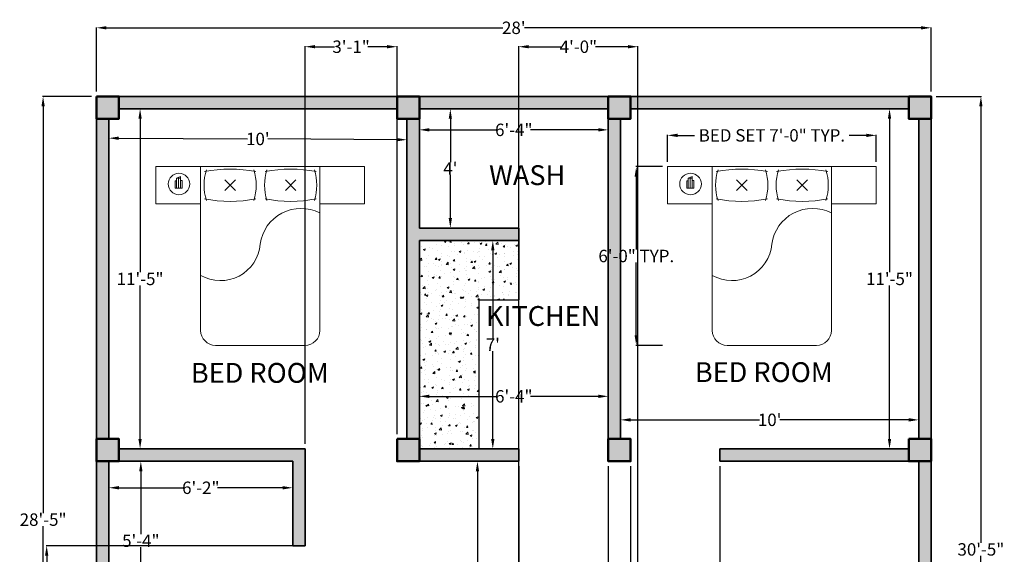
# Model space of a CAD drawing. Units: inches. Extents: x 157 to 553, y 100 to 520.
# Tile 2 of 2: x 157 to 553, y 304 to 520. Entities that reach past the tile are written whole.
import ezdxf

# ---------------------------------------------------------------- set-up
doc = ezdxf.new("R2010")
doc.units = ezdxf.units.IN
doc.header["$MEASUREMENT"] = 0
doc.layers.get('0').update_dxf_attribs({"color": 255})
for name, color, linetype, lineweight in [('A-ANNO-DIMS', 2, 'Continuous', 18), ('A-AREA-IDEN', 7, 'Continuous', 25), ('A-COLS', 7, 'Continuous', 50), ('A-FLOR-FIXT', 9, 'Continuous', 25), ('A-FLOR-FIXT-PATT', 252, 'Continuous', 13), ('A-FURN', 3, 'Continuous', 18), ('A-WALL', 7, 'Continuous', 35), ('A-WALL-PATT', 3, 'Continuous', 13)]:
    doc.layers.add(name, color=color, linetype=linetype, lineweight=lineweight)
doc.layers.add('A-COLS-PATT', color=18, linetype='Continuous', lineweight=13, true_color=0x000000)
doc.styles.get("Standard").update_dxf_attribs({"font": 'arial.ttf'})
doc.dimstyles.get("Standard").update_dxf_attribs({"dimtxt": 5, "dimasz": 4, "dimexe": 0.18, "dimexo": 2, "dimgap": 0.09, "dimtad": 0, "dimtih": 1, "dimtoh": 1, "dimdec": 0, "dimzin": 0, "dimdsep": 46, "dimlunit": 3, "dimtxsty": 'Standard', "dimcen": 2, "dimadec": 0, "dimazin": 0, "dimtfac": 1, "dimtdec": 0, "dimtofl": 0, "dimtmove": 0, "dimatfit": 3, "dimfxl": 1, "dimtolj": 1, "dimtzin": 0, "dimarcsym": 0})

# ---------------------------------------------------------------- blocks, each defined once
blk = doc.blocks.new('*D1')
at = {"layer": 'A-ANNO-DIMS', "color": 0, "lineweight": -2, "transparency": 16777216}
for p, q in [((187.79, 490.7), (187.79, 516.55)), ((191.79, 516.37), (351.41, 516.37)), ((519.79, 516.37), (360.16, 516.37)), ((523.79, 490.7), (523.79, 516.55))]:
    blk.add_line(p, q, dxfattribs=at)
at = {"layer": 'A-ANNO-DIMS', "color": 0, "transparency": 16777216}
for points in [[(191.79, 517.03), (191.79, 515.7), (187.79, 516.37)], [(519.79, 517.03), (519.79, 515.7), (523.79, 516.37)]]:
    blk.add_solid(points, dxfattribs=at)
at = {"layer": 'Defpoints', "color": 0, "transparency": 16777216}
for p in [(523.79, 516.37), (187.79, 488.7), (523.79, 488.7)]:
    blk.add_point(p, dxfattribs=at)
at = {"layer": 'A-ANNO-DIMS', "color": 0, "transparency": 16777216, "insert": (355.79, 516.37), "char_height": 5, "attachment_point": 5}
blk.add_mtext("\\A1;28'", dxfattribs=at)
blk = doc.blocks.new('*D2')
at = {"layer": 'A-ANNO-DIMS', "color": 0, "lineweight": -2, "transparency": 16777216}
for p, q in [((185.79, 488.7), (166.12, 488.7)), ((166.3, 484.7), (166.3, 320.85)), ((166.3, 151.7), (166.3, 315.56)), ((185.79, 147.7), (166.12, 147.7))]:
    blk.add_line(p, q, dxfattribs=at)
at = {"layer": 'A-ANNO-DIMS', "color": 0, "transparency": 16777216}
for points in [[(165.64, 484.7), (166.97, 484.7), (166.3, 488.7)], [(165.64, 151.7), (166.97, 151.7), (166.3, 147.7)]]:
    blk.add_solid(points, dxfattribs=at)
at = {"layer": 'Defpoints', "color": 0, "transparency": 16777216}
for p in [(187.79, 488.7), (166.3, 147.7), (187.79, 147.7)]:
    blk.add_point(p, dxfattribs=at)
at = {"layer": 'A-ANNO-DIMS', "color": 0, "transparency": 16777216, "insert": (166.3, 318.2), "char_height": 5, "attachment_point": 5}
blk.add_mtext('\\A1;28\'-5"', dxfattribs=at)
blk = doc.blocks.new('*D4')
at = {"layer": 'A-ANNO-DIMS', "color": 0, "lineweight": -2, "transparency": 16777216}
for p, q in [((512.79, 483.7), (506.88, 483.7)), ((507.06, 479.7), (507.06, 417.85)), ((507.06, 350.7), (507.06, 412.56)), ((512.79, 346.7), (506.88, 346.7))]:
    blk.add_line(p, q, dxfattribs=at)
at = {"layer": 'A-ANNO-DIMS', "color": 0, "transparency": 16777216}
for points in [[(506.39, 479.7), (507.72, 479.7), (507.06, 483.7)], [(506.39, 350.7), (507.72, 350.7), (507.06, 346.7)]]:
    blk.add_solid(points, dxfattribs=at)
at = {"layer": 'Defpoints', "color": 0, "transparency": 16777216}
for p in [(514.79, 483.7), (507.06, 346.7), (514.79, 346.7)]:
    blk.add_point(p, dxfattribs=at)
at = {"layer": 'A-ANNO-DIMS', "color": 0, "transparency": 16777216, "insert": (507.06, 415.2), "char_height": 5, "attachment_point": 5}
blk.add_mtext('\\A1;11\'-5"', dxfattribs=at)
blk = doc.blocks.new('*D5')
at = {"layer": 'A-ANNO-DIMS', "color": 0, "lineweight": -2, "transparency": 16777216}
for p, q in [((398.79, 352.7), (398.79, 358.58)), ((402.79, 358.4), (454.69, 358.4)), ((514.79, 358.4), (462.89, 358.4)), ((518.79, 352.7), (518.79, 358.58))]:
    blk.add_line(p, q, dxfattribs=at)
at = {"layer": 'A-ANNO-DIMS', "color": 0, "transparency": 16777216}
for points in [[(402.79, 359.07), (402.79, 357.73), (398.79, 358.4)], [(514.79, 359.07), (514.79, 357.73), (518.79, 358.4)]]:
    blk.add_solid(points, dxfattribs=at)
at = {"layer": 'Defpoints', "color": 0, "transparency": 16777216}
for p in [(518.79, 358.4), (398.79, 350.7), (518.79, 350.7)]:
    blk.add_point(p, dxfattribs=at)
at = {"layer": 'A-ANNO-DIMS', "color": 0, "transparency": 16777216, "insert": (458.79, 358.4), "char_height": 5, "attachment_point": 5}
blk.add_mtext("\\A1;10'", dxfattribs=at)
blk = doc.blocks.new('*D6')
at = {"layer": 'A-ANNO-DIMS', "color": 0, "lineweight": -2, "transparency": 16777216}
for p, q in [((198.79, 483.7), (205.52, 483.7)), ((205.34, 479.7), (205.34, 417.85)), ((205.34, 350.7), (205.34, 412.56)), ((198.79, 346.7), (205.52, 346.7))]:
    blk.add_line(p, q, dxfattribs=at)
at = {"layer": 'A-ANNO-DIMS', "color": 0, "transparency": 16777216}
for points in [[(204.67, 479.7), (206.01, 479.7), (205.34, 483.7)], [(204.67, 350.7), (206.01, 350.7), (205.34, 346.7)]]:
    blk.add_solid(points, dxfattribs=at)
at = {"layer": 'Defpoints', "color": 0, "transparency": 16777216}
for p in [(196.79, 483.7), (196.79, 346.7), (205.34, 346.7)]:
    blk.add_point(p, dxfattribs=at)
at = {"layer": 'A-ANNO-DIMS', "color": 0, "transparency": 16777216, "insert": (205.34, 415.2), "char_height": 5, "attachment_point": 5}
blk.add_mtext('\\A1;11\'-5"', dxfattribs=at)
blk = doc.blocks.new('*D7')
at = {"layer": 'A-ANNO-DIMS', "color": 0, "lineweight": -2, "transparency": 16777216}
for p, q in [((192.78, 477.7), (192.75, 471.72)), ((312.78, 477.08), (312.75, 471.09)), ((196.75, 471.88), (248.65, 471.61)), ((308.75, 471.3), (256.84, 471.57))]:
    blk.add_line(p, q, dxfattribs=at)
at = {"layer": 'A-ANNO-DIMS', "color": 0, "transparency": 16777216}
for points in [[(196.75, 472.55), (196.74, 471.21), (192.75, 471.9)], [(308.75, 471.96), (308.74, 470.63), (312.75, 471.27)]]:
    blk.add_solid(points, dxfattribs=at)
at = {"layer": 'Defpoints', "color": 0, "transparency": 16777216}
for p in [(192.79, 479.7), (312.79, 479.08), (312.75, 471.27)]:
    blk.add_point(p, dxfattribs=at)
at = {"layer": 'A-ANNO-DIMS', "color": 0, "transparency": 16777216, "insert": (252.75, 471.59), "char_height": 5, "attachment_point": 5}
blk.add_mtext("\\A1;10'", dxfattribs=at)
blk = doc.blocks.new('*D8')
at = {"layer": 'A-ANNO-DIMS', "color": 0, "lineweight": -2, "transparency": 16777216}
for p, q in [((317.79, 477.7), (317.79, 475.08)), ((393.79, 477.7), (393.79, 475.08)), ((321.79, 475.26), (349.04, 475.26)), ((389.79, 475.26), (362.54, 475.26))]:
    blk.add_line(p, q, dxfattribs=at)
at = {"layer": 'A-ANNO-DIMS', "color": 0, "transparency": 16777216}
for points in [[(321.79, 475.93), (321.79, 474.59), (317.79, 475.26)], [(389.79, 475.93), (389.79, 474.59), (393.79, 475.26)]]:
    blk.add_solid(points, dxfattribs=at)
at = {"layer": 'Defpoints', "color": 0, "transparency": 16777216}
for p in [(317.79, 479.7), (393.79, 479.7), (393.79, 475.26)]:
    blk.add_point(p, dxfattribs=at)
at = {"layer": 'A-ANNO-DIMS', "color": 0, "transparency": 16777216, "insert": (355.79, 475.26), "char_height": 5, "attachment_point": 5}
blk.add_mtext('\\A1;6\'-4"', dxfattribs=at)
blk = doc.blocks.new('*D9')
at = {"layer": 'A-ANNO-DIMS', "color": 0, "lineweight": -2, "transparency": 16777216}
for p, q in [((319.79, 483.7), (330.43, 483.7)), ((330.25, 479.7), (330.25, 462.29)), ((330.25, 439.7), (330.25, 457.11)), ((319.79, 435.7), (330.43, 435.7))]:
    blk.add_line(p, q, dxfattribs=at)
at = {"layer": 'A-ANNO-DIMS', "color": 0, "transparency": 16777216}
for points in [[(329.58, 479.7), (330.91, 479.7), (330.25, 483.7)], [(329.58, 439.7), (330.91, 439.7), (330.25, 435.7)]]:
    blk.add_solid(points, dxfattribs=at)
at = {"layer": 'Defpoints', "color": 0, "transparency": 16777216}
for p in [(317.79, 483.7), (330.25, 483.7), (317.79, 435.7)]:
    blk.add_point(p, dxfattribs=at)
at = {"layer": 'A-ANNO-DIMS', "color": 0, "transparency": 16777216, "insert": (330.25, 459.7), "char_height": 5, "attachment_point": 5}
blk.add_mtext("\\A1;4'", dxfattribs=at)
blk = doc.blocks.new('*D10')
at = {"layer": 'A-ANNO-DIMS', "color": 0, "lineweight": -2, "transparency": 16777216}
for p, q in [((339.59, 430.7), (347.52, 430.7)), ((347.34, 426.7), (347.34, 391.29)), ((347.34, 350.7), (347.34, 386.11)), ((339.59, 346.7), (347.52, 346.7))]:
    blk.add_line(p, q, dxfattribs=at)
at = {"layer": 'A-ANNO-DIMS', "color": 0, "transparency": 16777216}
for points in [[(346.67, 426.7), (348, 426.7), (347.34, 430.7)], [(346.67, 350.7), (348, 350.7), (347.34, 346.7)]]:
    blk.add_solid(points, dxfattribs=at)
at = {"layer": 'Defpoints', "color": 0, "transparency": 16777216}
for p in [(337.59, 430.7), (347.34, 430.7), (337.59, 346.7)]:
    blk.add_point(p, dxfattribs=at)
at = {"layer": 'A-ANNO-DIMS', "color": 0, "transparency": 16777216, "insert": (347.34, 388.7), "char_height": 5, "attachment_point": 5}
blk.add_mtext("\\A1;7'", dxfattribs=at)
blk = doc.blocks.new('*D11')
at = {"layer": 'A-ANNO-DIMS', "color": 0, "lineweight": -2, "transparency": 16777216}
for p, q in [((317.79, 375.65), (317.79, 367.7)), ((393.79, 375.65), (393.79, 367.7)), ((321.79, 367.88), (349.04, 367.88)), ((389.79, 367.88), (362.54, 367.88))]:
    blk.add_line(p, q, dxfattribs=at)
at = {"layer": 'A-ANNO-DIMS', "color": 0, "transparency": 16777216}
for points in [[(321.79, 368.55), (321.79, 367.21), (317.79, 367.88)], [(389.79, 368.55), (389.79, 367.21), (393.79, 367.88)]]:
    blk.add_solid(points, dxfattribs=at)
at = {"layer": 'Defpoints', "color": 0, "transparency": 16777216}
for p in [(317.79, 377.65), (393.79, 377.65), (393.79, 367.88)]:
    blk.add_point(p, dxfattribs=at)
at = {"layer": 'A-ANNO-DIMS', "color": 0, "transparency": 16777216, "insert": (355.79, 367.88), "char_height": 5, "attachment_point": 5}
blk.add_mtext('\\A1;6\'-4"', dxfattribs=at)
blk = doc.blocks.new('*D12')
at = {"layer": 'A-ANNO-DIMS', "color": 0, "lineweight": -2, "transparency": 16777216}
for p, q in [((192.79, 339.7), (192.79, 330.86)), ((266.79, 339.7), (266.79, 330.86)), ((196.79, 331.04), (223.04, 331.04)), ((262.79, 331.04), (236.54, 331.04))]:
    blk.add_line(p, q, dxfattribs=at)
at = {"layer": 'A-ANNO-DIMS', "color": 0, "transparency": 16777216}
for points in [[(196.79, 331.71), (196.79, 330.37), (192.79, 331.04)], [(262.79, 331.71), (262.79, 330.37), (266.79, 331.04)]]:
    blk.add_solid(points, dxfattribs=at)
at = {"layer": 'Defpoints', "color": 0, "transparency": 16777216}
for p in [(192.79, 341.7), (266.79, 341.7), (266.79, 331.04)]:
    blk.add_point(p, dxfattribs=at)
at = {"layer": 'A-ANNO-DIMS', "color": 0, "transparency": 16777216, "insert": (229.79, 331.04), "char_height": 5, "attachment_point": 5}
blk.add_mtext('\\A1;6\'-2"', dxfattribs=at)
blk = doc.blocks.new('*D13')
at = {"layer": 'A-ANNO-DIMS', "color": 0, "lineweight": -2, "transparency": 16777216}
for p, q in [((198.79, 341.7), (205.83, 341.7)), ((205.65, 337.7), (205.65, 312.34)), ((205.65, 281.7), (205.65, 307.07)), ((198.79, 277.7), (205.83, 277.7))]:
    blk.add_line(p, q, dxfattribs=at)
at = {"layer": 'A-ANNO-DIMS', "color": 0, "transparency": 16777216}
for points in [[(204.99, 337.7), (206.32, 337.7), (205.65, 341.7)], [(204.99, 281.7), (206.32, 281.7), (205.65, 277.7)]]:
    blk.add_solid(points, dxfattribs=at)
at = {"layer": 'Defpoints', "color": 0, "transparency": 16777216}
for p in [(196.79, 341.7), (196.79, 277.7), (205.65, 277.7)]:
    blk.add_point(p, dxfattribs=at)
at = {"layer": 'A-ANNO-DIMS', "color": 0, "transparency": 16777216, "insert": (205.65, 309.7), "char_height": 5, "attachment_point": 5}
blk.add_mtext('\\A1;5\'-4"', dxfattribs=at)
blk = doc.blocks.new('*D18')
at = {"layer": 'A-ANNO-DIMS', "color": 0, "lineweight": -2, "transparency": 16777216}
for p, q in [((355.79, 341.7), (340.98, 341.7)), ((341.16, 337.7), (341.16, 285.85)), ((341.16, 228.7), (341.16, 280.56)), ((355.79, 224.7), (340.98, 224.7))]:
    blk.add_line(p, q, dxfattribs=at)
at = {"layer": 'A-ANNO-DIMS', "color": 0, "transparency": 16777216}
for points in [[(340.49, 337.7), (341.82, 337.7), (341.16, 341.7)], [(340.49, 228.7), (341.82, 228.7), (341.16, 224.7)]]:
    blk.add_solid(points, dxfattribs=at)
at = {"layer": 'Defpoints', "color": 0, "transparency": 16777216}
for p in [(341.16, 341.7), (357.79, 341.7), (357.79, 224.7)]:
    blk.add_point(p, dxfattribs=at)
at = {"layer": 'A-ANNO-DIMS', "color": 0, "transparency": 16777216, "insert": (341.16, 283.2), "char_height": 5, "attachment_point": 5}
blk.add_mtext('\\A1;9\'-9"', dxfattribs=at)
blk = doc.blocks.new('BED-DOUBLE-WITH-NIGHTSTANDS')
for p, q in [((0, 72), (18, 72)), ((0, 57), (0, 72)), ((6, 72), (84, 72)), ((18, 72), (18, 6)), ((66, 6), (66, 72)), ((84, 72), (84, 57)), ((9.95, 67.98), (8.32, 67.38)), ((9.95, 67.38), (9.95, 67.98)), ((9.14, 67.38), (9.14, 63.35)), ((32, 66.63), (27.75, 62.4)), ((27.76, 66.64), (31.99, 62.39)), ((56.35, 66.63), (52.1, 62.4)), ((52.11, 66.64), (56.34, 62.39)), ((18, 57), (0, 57)), ((84, 57), (66, 57)), ((24, 0), (60, 0))]:
    blk.add_line(p, q)
for points in [[(8.32, 63.35), (7.8, 63.35), (7.8, 66.31), (8.32, 66.31)], [(8.32, 63.35), (9.95, 63.35), (9.95, 67.38), (8.32, 67.38)], [(9.95, 63.35), (10.59, 63.35), (10.59, 66.42), (9.95, 66.42)]]:
    blk.add_lwpolyline(points, close=True)
blk.add_circle((9.27, 65.01), 4.35)
for centre, radius, start, end in [((54.23, 16.39), 56.63, 100.869, 100.8807), ((54.23, 16.39), 56.63, 79.1193, 79.131), ((40, 64.52), 20.63, 162.5077, 197.4923), ((29.88, 16.39), 54.63, 79.1193, 100.8807), ((19.75, 64.52), 20.62, 342.5077, 17.4923), ((64.35, 64.52), 20.63, 162.5077, 197.4923), ((54.23, 16.39), 54.63, 79.1193, 100.8807), ((44.1, 64.52), 20.62, 342.5077, 17.4923), ((29.88, 112.64), 54.63, 259.1193, 280.8807), ((54.23, 112.64), 54.63, 259.1193, 280.8807), ((58.39, 38.66), 16.52, 62.5747, 172.7011), ((25.97, 42.18), 16.1, 240.3431, 354.9328), ((24, 6), 6, 180, 270), ((60, 6), 6, 270, 0)]:
    blk.add_arc(centre, radius, start, end)
blk = doc.blocks.new('*D21')
at = {"layer": 'A-ANNO-DIMS', "color": 0, "lineweight": -2, "transparency": 16777216}
for p, q in [((417.7, 462.43), (417.7, 473.21)), ((421.7, 473.03), (428.56, 473.03)), ((497.7, 473.03), (490.83, 473.03)), ((501.7, 462.43), (501.7, 473.21))]:
    blk.add_line(p, q, dxfattribs=at)
at = {"layer": 'A-ANNO-DIMS', "color": 0, "transparency": 16777216}
for points in [[(421.7, 473.7), (421.7, 472.36), (417.7, 473.03)], [(497.7, 473.7), (497.7, 472.36), (501.7, 473.03)]]:
    blk.add_solid(points, dxfattribs=at)
at = {"layer": 'Defpoints', "color": 0, "transparency": 16777216}
for p in [(501.7, 473.03), (417.7, 460.43), (501.7, 460.43)]:
    blk.add_point(p, dxfattribs=at)
at = {"layer": 'A-ANNO-DIMS', "color": 0, "transparency": 16777216, "insert": (459.7, 473.03), "char_height": 5, "attachment_point": 5}
blk.add_mtext('\\A1;BED SET 7\'-0" TYP.', dxfattribs=at)
blk = doc.blocks.new('*D22')
at = {"layer": 'A-ANNO-DIMS', "color": 0, "lineweight": -2, "transparency": 16777216}
for p, q in [((415.7, 460.43), (404.92, 460.43)), ((405.1, 456.43), (405.1, 427.07)), ((405.1, 392.43), (405.1, 421.79)), ((415.7, 388.43), (404.92, 388.43))]:
    blk.add_line(p, q, dxfattribs=at)
at = {"layer": 'A-ANNO-DIMS', "color": 0, "transparency": 16777216}
for points in [[(404.43, 456.43), (405.76, 456.43), (405.1, 460.43)], [(404.43, 392.43), (405.76, 392.43), (405.1, 388.43)]]:
    blk.add_solid(points, dxfattribs=at)
at = {"layer": 'Defpoints', "color": 0, "transparency": 16777216}
for p in [(405.1, 460.43), (417.7, 460.43), (417.7, 388.43)]:
    blk.add_point(p, dxfattribs=at)
at = {"layer": 'A-ANNO-DIMS', "color": 0, "transparency": 16777216, "insert": (405.1, 424.43), "char_height": 5, "attachment_point": 5}
blk.add_mtext('\\A1;6\'-0" TYP.', dxfattribs=at)
blk = doc.blocks.new('*D23')
at = {"layer": 'A-ANNO-DIMS', "color": 0, "lineweight": -2, "transparency": 16777216}
for p, q in [((525.79, 488.7), (544.02, 488.7)), ((543.84, 484.7), (543.84, 308.85)), ((543.84, 127.7), (543.84, 303.56)), ((406.79, 123.7), (544.02, 123.7))]:
    blk.add_line(p, q, dxfattribs=at)
at = {"layer": 'A-ANNO-DIMS', "color": 0, "transparency": 16777216}
for points in [[(543.17, 484.7), (544.5, 484.7), (543.84, 488.7)], [(543.17, 127.7), (544.5, 127.7), (543.84, 123.7)]]:
    blk.add_solid(points, dxfattribs=at)
at = {"layer": 'Defpoints', "color": 0, "transparency": 16777216}
for p in [(523.79, 488.7), (404.79, 123.7), (543.84, 123.7)]:
    blk.add_point(p, dxfattribs=at)
at = {"layer": 'A-ANNO-DIMS', "color": 0, "transparency": 16777216, "insert": (543.84, 306.2), "char_height": 5, "attachment_point": 5}
blk.add_mtext('\\A1;30\'-5"', dxfattribs=at)
blk = doc.blocks.new('*D24')
at = {"layer": 'A-ANNO-DIMS', "color": 0, "lineweight": -2, "transparency": 16777216}
for p, q in [((271.79, 348.7), (271.79, 508.93)), ((275.79, 508.75), (283.55, 508.75)), ((304.79, 508.75), (297.02, 508.75)), ((308.79, 352.7), (308.79, 508.93))]:
    blk.add_line(p, q, dxfattribs=at)
at = {"layer": 'A-ANNO-DIMS', "color": 0, "transparency": 16777216}
for points in [[(275.79, 509.42), (275.79, 508.09), (271.79, 508.75)], [(304.79, 509.42), (304.79, 508.09), (308.79, 508.75)]]:
    blk.add_solid(points, dxfattribs=at)
at = {"layer": 'Defpoints', "color": 0, "transparency": 16777216}
for p in [(308.79, 508.75), (308.79, 350.7), (271.79, 346.7)]:
    blk.add_point(p, dxfattribs=at)
at = {"layer": 'A-ANNO-DIMS', "color": 0, "transparency": 16777216, "insert": (290.29, 508.75), "char_height": 5, "attachment_point": 5}
blk.add_mtext('\\A1;3\'-1"', dxfattribs=at)
blk = doc.blocks.new('*D25')
at = {"layer": 'A-ANNO-DIMS', "color": 0, "lineweight": -2, "transparency": 16777216}
for p, q in [((357.79, 339.7), (357.79, 103.47)), ((393.79, 339.7), (393.79, 103.47)), ((361.79, 103.65), (369.05, 103.65)), ((389.79, 103.65), (382.52, 103.65))]:
    blk.add_line(p, q, dxfattribs=at)
at = {"layer": 'A-ANNO-DIMS', "color": 0, "transparency": 16777216}
for points in [[(361.79, 104.32), (361.79, 102.99), (357.79, 103.65)], [(389.79, 104.32), (389.79, 102.99), (393.79, 103.65)]]:
    blk.add_solid(points, dxfattribs=at)
at = {"layer": 'Defpoints', "color": 0, "transparency": 16777216}
for p in [(357.79, 341.7), (393.79, 341.7), (393.79, 103.65)]:
    blk.add_point(p, dxfattribs=at)
at = {"layer": 'A-ANNO-DIMS', "color": 0, "transparency": 16777216, "insert": (375.79, 103.65), "char_height": 5, "attachment_point": 5}
blk.add_mtext('\\A1;3\'-0"', dxfattribs=at)
blk = doc.blocks.new('*D26')
at = {"layer": 'A-ANNO-DIMS', "color": 0, "lineweight": -2, "transparency": 16777216}
for p, q in [((402.79, 339.7), (402.79, 103.47)), ((438.79, 339.7), (438.79, 103.47)), ((406.79, 103.65), (414.05, 103.65)), ((434.79, 103.65), (427.52, 103.65))]:
    blk.add_line(p, q, dxfattribs=at)
at = {"layer": 'A-ANNO-DIMS', "color": 0, "transparency": 16777216}
for points in [[(406.79, 104.32), (406.79, 102.99), (402.79, 103.65)], [(434.79, 104.32), (434.79, 102.99), (438.79, 103.65)]]:
    blk.add_solid(points, dxfattribs=at)
at = {"layer": 'Defpoints', "color": 0, "transparency": 16777216}
for p in [(402.79, 341.7), (438.79, 341.7), (438.79, 103.65)]:
    blk.add_point(p, dxfattribs=at)
at = {"layer": 'A-ANNO-DIMS', "color": 0, "transparency": 16777216, "insert": (420.79, 103.65), "char_height": 5, "attachment_point": 5}
blk.add_mtext('\\A1;3\'-0"', dxfattribs=at)
blk = doc.blocks.new('*D27')
at = {"layer": 'A-ANNO-DIMS', "color": 0, "lineweight": -2, "transparency": 16777216}
for p, q in [((269.79, 307.7), (167.56, 307.7)), ((167.74, 303.7), (167.74, 295.35)), ((167.74, 281.7), (167.74, 290.06)), ((306.79, 277.7), (167.56, 277.7))]:
    blk.add_line(p, q, dxfattribs=at)
at = {"layer": 'A-ANNO-DIMS', "color": 0, "transparency": 16777216}
for points in [[(167.07, 303.7), (168.4, 303.7), (167.74, 307.7)], [(167.07, 281.7), (168.4, 281.7), (167.74, 277.7)]]:
    blk.add_solid(points, dxfattribs=at)
at = {"layer": 'Defpoints', "color": 0, "transparency": 16777216}
for p in [(271.79, 307.7), (167.74, 277.7), (308.79, 277.7)]:
    blk.add_point(p, dxfattribs=at)
at = {"layer": 'A-ANNO-DIMS', "color": 0, "transparency": 16777216, "insert": (167.74, 292.7), "char_height": 5, "attachment_point": 5}
blk.add_mtext('\\A1;2\'-6"', dxfattribs=at)
blk = doc.blocks.new('*D29')
at = {"layer": 'A-ANNO-DIMS', "color": 0, "lineweight": -2, "transparency": 16777216}
for p, q in [((357.79, 226.7), (357.79, 508.93)), ((361.79, 508.75), (374.95, 508.75)), ((401.79, 508.75), (388.62, 508.75)), ((405.79, 226.7), (405.79, 508.93))]:
    blk.add_line(p, q, dxfattribs=at)
at = {"layer": 'A-ANNO-DIMS', "color": 0, "transparency": 16777216}
for points in [[(361.79, 509.42), (361.79, 508.09), (357.79, 508.75)], [(401.79, 509.42), (401.79, 508.09), (405.79, 508.75)]]:
    blk.add_solid(points, dxfattribs=at)
at = {"layer": 'Defpoints', "color": 0, "transparency": 16777216}
for p in [(405.79, 508.75), (357.79, 224.7), (405.79, 224.7)]:
    blk.add_point(p, dxfattribs=at)
at = {"layer": 'A-ANNO-DIMS', "color": 0, "transparency": 16777216, "insert": (381.79, 508.75), "char_height": 5, "attachment_point": 5}
blk.add_mtext('\\A1;4\'-0"', dxfattribs=at)

msp = doc.modelspace()

# ---------------------------------------------------------------- hatches: boundary and pattern name
at = {"layer": 'A-COLS-PATT'}
h = msp.add_hatch(color=256, dxfattribs=at)
h.dxf.hatch_style = 1
h.paths.add_polyline_path([(196.79, 156.7), (187.79, 156.7), (187.79, 147.7), (196.79, 147.7)])
h.paths.add_polyline_path([(317.79, 156.7), (308.79, 156.7), (308.79, 147.7), (317.79, 147.7)])
h.paths.add_polyline_path([(440.79, 156.7), (431.79, 156.7), (431.79, 147.7), (440.79, 147.7)])
h.paths.add_polyline_path([(523.79, 156.7), (514.79, 156.7), (514.79, 147.7), (523.79, 147.7)])
h.paths.add_polyline_path([(523.79, 277.7), (514.79, 277.7), (514.79, 268.7), (523.79, 268.7)])
h.paths.add_polyline_path([(440.79, 277.7), (431.79, 277.7), (431.79, 268.7), (440.79, 268.7)])
h.paths.add_polyline_path([(317.79, 277.7), (308.79, 277.7), (308.79, 268.7), (317.79, 268.7)])
h.paths.add_polyline_path([(196.79, 350.7), (187.79, 350.7), (187.79, 341.7), (196.79, 341.7)])
h.paths.add_polyline_path([(317.79, 350.7), (308.79, 350.7), (308.79, 341.7), (317.79, 341.7)])
h.paths.add_polyline_path([(402.79, 350.7), (393.79, 350.7), (393.79, 341.7), (402.79, 341.7)])
h.paths.add_polyline_path([(523.79, 350.7), (514.79, 350.7), (514.79, 341.7), (523.79, 341.7)])
h.paths.add_polyline_path([(523.79, 488.7), (514.79, 488.7), (514.79, 479.7), (523.79, 479.7)])
h.paths.add_polyline_path([(402.79, 488.7), (393.79, 488.7), (393.79, 479.7), (402.79, 479.7)])
h.paths.add_polyline_path([(317.79, 488.7), (308.79, 488.7), (308.79, 479.7), (317.79, 479.7)])
h.paths.add_polyline_path([(196.79, 488.7), (187.79, 488.7), (187.79, 479.7), (196.79, 479.7)])
at = {"layer": 'A-FLOR-FIXT-PATT'}
h = msp.add_hatch(dxfattribs=at)
h.set_pattern_fill('AR-CONC', color=256)
h.set_pattern_definition([(50, (0, 0), (7.1726, -0.62752), [0.75, -8.25]), (355, (0, 0), (-1.38751, 7.52192), [0.6, -6.6]), (100.4514, (0.598, -0.052), (5.78509, 6.8944), [0.6374, -7.01142]), (46.1842, (0, 2), (10.67241, -1.65519), [1.125, -12.375]), (96.6356, (0.889, 1.862), (9.34662, 9.74119), [0.9561, -10.51714]), (351.1842, (0, 2), (9.34662, 9.74119), [0.9, -9.9]), (21, (1, 1.5), (5.96907, -4.02619), [0.75, -8.25]), (326, (1, 1.5), (2.43315, 7.2515), [0.6, -6.6]), (71.4514, (1.4974, 1.1645), (8.40222, 3.22531), [0.6374, -7.01142]), (37.5, (0, 0), (0.121599, 3.328939), [0, -6.52, 0, -6.7, 0, -6.625]), (7.5, (0, 0), (2.630695, 3.944117), [0, -3.82, 0, -6.37, 0, -2.525]), (327.5, (-2.23, 0), (5.338224, -0.225549), [0, -2.5, 0, -7.8, 0, -10.35]), (317.5, (-3.23, 0), (5.83186, 1.00105), [0, -3.25, 0, -5.18, 0, -7.35])])
h.paths.add_polyline_path([(357.79, 430.7), (317.79, 430.7), (317.79, 346.7), (341.79, 346.7), (341.79, 406.7), (357.79, 406.7)])
at = {"layer": 'A-WALL-PATT'}
h = msp.add_hatch(color=256, dxfattribs=at)
h.dxf.hatch_style = 1
h.paths.add_polyline_path([(271.79, 346.7), (196.79, 346.7), (196.79, 341.7), (266.79, 341.7), (266.79, 307.7), (271.79, 307.7)])
h.paths.add_polyline_path([(308.79, 277.7), (192.79, 277.7), (192.79, 341.7), (187.79, 341.7), (187.79, 156.7), (192.79, 156.7), (192.79, 272.7), (308.79, 272.7)])
h.paths.add_polyline_path([(357.79, 224.7), (317.79, 224.7), (317.79, 232.7), (312.79, 232.7), (312.79, 156.7), (317.79, 156.7), (317.79, 219.7), (357.79, 219.7)])
h.paths.add_polyline_path([(308.79, 152.7), (196.79, 152.7), (196.79, 147.7), (308.79, 147.7)])
h.paths.add_polyline_path([(440.79, 268.7), (435.79, 268.7), (435.79, 224.7), (405.79, 224.7), (405.79, 219.7), (435.79, 219.7), (435.79, 156.7), (440.79, 156.7)])
h.paths.add_polyline_path([(523.79, 147.7), (518.79, 147.7), (518.79, 131.7), (440.79, 131.7), (440.79, 147.7), (435.79, 147.7), (435.79, 126.7), (523.79, 126.7)])
h.paths.add_polyline_path([(523.79, 268.7), (518.79, 268.7), (518.79, 156.7), (523.79, 156.7)])
h.paths.add_polyline_path([(523.79, 341.7), (518.79, 341.7), (518.79, 277.7), (523.79, 277.7)])
h.paths.add_polyline_path([(523.79, 479.7), (518.79, 479.7), (518.79, 350.7), (523.79, 350.7)])
h.paths.add_polyline_path([(514.79, 346.7), (438.79, 346.7), (438.79, 341.7), (514.79, 341.7)])
h.paths.add_polyline_path([(317.79, 430.7), (357.79, 430.7), (357.79, 435.7), (317.79, 435.7), (317.79, 479.7), (312.79, 479.7), (312.79, 350.7), (317.79, 350.7)])
h.paths.add_polyline_path([(357.79, 346.7), (317.79, 346.7), (317.79, 341.7), (357.79, 341.7)])
h.paths.add_polyline_path([(398.79, 479.7), (393.79, 479.7), (393.79, 350.7), (398.79, 350.7)])
h.paths.add_polyline_path([(192.79, 479.7), (187.79, 479.7), (187.79, 350.7), (192.79, 350.7)])
h.paths.add_polyline_path([(308.79, 488.7), (196.79, 488.7), (196.79, 483.7), (308.79, 483.7)])
h.paths.add_polyline_path([(393.79, 488.7), (317.79, 488.7), (317.79, 483.7), (393.79, 483.7)])
h.paths.add_polyline_path([(514.79, 488.7), (402.79, 488.7), (402.79, 483.7), (514.79, 483.7)])

# ---------------------------------------------------------------- linework, layer by layer
at = {"layer": 'A-COLS'}
for points in [[(187.79, 488.7), (196.79, 488.7), (196.79, 479.7), (187.79, 479.7)], [(308.79, 488.7), (317.79, 488.7), (317.79, 479.7), (308.79, 479.7)], [(393.79, 488.7), (402.79, 488.7), (402.79, 479.7), (393.79, 479.7)], [(514.79, 488.7), (523.79, 488.7), (523.79, 479.7), (514.79, 479.7)], [(187.79, 350.7), (196.79, 350.7), (196.79, 341.7), (187.79, 341.7)], [(308.79, 350.7), (317.79, 350.7), (317.79, 341.7), (308.79, 341.7)], [(393.79, 350.7), (402.79, 350.7), (402.79, 341.7), (393.79, 341.7)], [(514.79, 350.7), (523.79, 350.7), (523.79, 341.7), (514.79, 341.7)]]:
    msp.add_lwpolyline(points, close=True, dxfattribs=at)
at = {"layer": 'A-FLOR-FIXT'}
for p, q in [((357.79, 430.7), (357.79, 406.7)), ((341.79, 406.7), (357.79, 406.7)), ((341.79, 346.7), (341.79, 406.7))]:
    msp.add_line(p, q, dxfattribs=at)
at = {"layer": 'A-WALL'}
for p, q in [((187.79, 488.7), (523.79, 488.7)), ((187.79, 147.7), (187.79, 488.7)), ((317.79, 435.7), (317.79, 488.7)), ((393.79, 341.7), (393.79, 488.7)), ((523.79, 488.7), (523.79, 147.7)), ((196.79, 483.7), (308.79, 483.7)), ((317.79, 483.7), (393.79, 483.7)), ((402.79, 483.7), (514.79, 483.7)), ((192.79, 350.7), (192.79, 479.7)), ((312.79, 350.7), (312.79, 479.7)), ((398.79, 350.7), (398.79, 479.7)), ((518.79, 350.7), (518.79, 479.7)), ((317.79, 435.7), (357.79, 435.7)), ((357.79, 435.7), (357.79, 430.7)), ((317.79, 341.7), (317.79, 430.7)), ((317.79, 430.7), (357.79, 430.7)), ((196.79, 346.7), (271.79, 346.7)), ((271.79, 307.7), (271.79, 346.7)), ((317.79, 346.7), (357.79, 346.7)), ((357.79, 346.7), (357.79, 341.7)), ((438.79, 346.7), (514.79, 346.7)), ((438.79, 341.7), (438.79, 346.7)), ((187.79, 341.7), (266.79, 341.7)), ((192.79, 277.7), (192.79, 341.7)), ((266.79, 307.7), (266.79, 341.7)), ((308.79, 341.7), (357.79, 341.7)), ((393.79, 341.7), (402.79, 341.7)), ((438.79, 341.7), (523.79, 341.7)), ((518.79, 277.7), (518.79, 341.7)), ((266.79, 307.7), (271.79, 307.7))]:
    msp.add_line(p, q, dxfattribs=at)

# ---------------------------------------------------------------- block references
at = {"layer": 'A-FURN'}
for p in [(211.73, 388.43), (417.69, 388.43)]:
    msp.add_blockref('BED-DOUBLE-WITH-NIGHTSTANDS', p, dxfattribs=at)

# ---------------------------------------------------------------- texts
at = {"layer": 'A-AREA-IDEN', "char_height": 8, "attachment_point": 1}
for s, insert in [('{WASH}', (345.84, 460.99)), ('{KITCHEN}', (344.6, 404.25)), ('{BED ROOM}', (225.8, 381.33)), ('{BED ROOM}', (428.7, 381.62))]:
    msp.add_mtext_dynamic_manual_height_columns(s, width=68.988, gutter_width=1, heights=[0], dxfattribs=dict(at, insert=insert))

# ---------------------------------------------------------------- dimensions: what is measured, and where the dimension line sits
at = {"layer": 'A-ANNO-DIMS'}
for base, p1, p2, override, picture, middle in [((523.79, 516.37), (187.79, 488.7), (523.79, 488.7), {"dimclrd": 0, "dimclre": 0, "dimclrt": 0}, '*D1', (355.79, 516.37)), ((308.79, 508.75), (271.79, 346.7), (308.79, 350.7), {"dimdec": 1, "dimlfac": 1, "dimrnd": 0, "dimzin": 1, "dimdsep": 46, "dimlunit": 4, "dimfrac": 2}, '*D24', (290.29, 508.75)), ((405.79, 508.75), (357.79, 224.7), (405.79, 224.7), {"dimdec": 1, "dimlfac": 1, "dimrnd": 0, "dimzin": 1, "dimdsep": 46, "dimlunit": 4, "dimfrac": 2}, '*D29', (381.79, 508.75)), ((393.79, 475.26), (317.79, 479.7), (393.79, 479.7), {"dimclrd": 0, "dimclre": 0, "dimclrt": 0}, '*D8', (355.79, 475.26)), ((393.79, 367.88), (317.79, 377.65), (393.79, 377.65), {"dimclrd": 0, "dimclre": 0, "dimclrt": 0}, '*D11', (355.79, 367.88)), ((518.79, 358.4), (398.79, 350.7), (518.79, 350.7), {"dimclrd": 0, "dimclre": 0, "dimclrt": 0}, '*D5', (458.79, 358.4)), ((266.79, 331.04), (192.79, 341.7), (266.79, 341.7), {"dimclrd": 0, "dimclre": 0, "dimclrt": 0}, '*D12', (229.79, 331.04)), ((393.79, 103.65), (357.79, 341.7), (393.79, 341.7), {"dimdec": 1, "dimlfac": 1, "dimrnd": 0, "dimzin": 1, "dimdsep": 46, "dimlunit": 4, "dimfrac": 2}, '*D25', (375.79, 103.65)), ((438.79, 103.65), (402.79, 341.7), (438.79, 341.7), {"dimdec": 1, "dimlfac": 1, "dimrnd": 0, "dimzin": 1, "dimdsep": 46, "dimlunit": 4, "dimfrac": 2}, '*D26', (420.79, 103.65))]:
    dim = msp.add_linear_dim(base=base, p1=p1, p2=p2, dimstyle='Standard', override=override, dxfattribs=at)
    dim.commit()
    dim.dimension.update_dxf_attribs({"geometry": picture, "text_midpoint": middle})
for base, p1, p2, override, picture, middle in [((166.3, 147.7), (187.79, 488.7), (187.79, 147.7), {"dimclrd": 0, "dimclre": 0, "dimclrt": 0}, '*D2', (166.3, 318.2)), ((543.84, 123.7), (523.79, 488.7), (404.79, 123.7), {"dimdec": 1, "dimlfac": 1, "dimrnd": 0, "dimzin": 1, "dimdsep": 46, "dimlunit": 4, "dimfrac": 2}, '*D23', (543.84, 306.2)), ((205.34, 346.7), (196.79, 483.7), (196.79, 346.7), {"dimclrd": 0, "dimclre": 0, "dimclrt": 0}, '*D6', (205.34, 415.2)), ((330.25, 483.7), (317.79, 435.7), (317.79, 483.7), {"dimclrd": 0, "dimclre": 0, "dimclrt": 0}, '*D9', (330.25, 459.7)), ((507.06, 346.7), (514.79, 483.7), (514.79, 346.7), {"dimclrd": 0, "dimclre": 0, "dimclrt": 0}, '*D4', (507.06, 415.2)), ((347.34, 430.7), (337.59, 346.7), (337.59, 430.7), {"dimclrd": 0, "dimclre": 0, "dimclrt": 0}, '*D10', (347.34, 388.7)), ((205.65, 277.7), (196.79, 341.7), (196.79, 277.7), {"dimclrd": 0, "dimclre": 0, "dimclrt": 0}, '*D13', (205.65, 309.7)), ((341.16, 341.7), (357.79, 224.7), (357.79, 341.7), {"dimclrd": 0, "dimclre": 0, "dimclrt": 0}, '*D18', (341.16, 283.2)), ((167.74, 277.7), (271.79, 307.7), (308.79, 277.7), {"dimdec": 1, "dimlfac": 1, "dimrnd": 0, "dimzin": 1, "dimdsep": 46, "dimlunit": 4, "dimfrac": 2}, '*D27', (167.74, 292.7))]:
    dim = msp.add_linear_dim(base=base, p1=p1, p2=p2, angle=90, dimstyle='Standard', override=override, dxfattribs=at)
    dim.commit()
    dim.dimension.update_dxf_attribs({"geometry": picture, "text_midpoint": middle})
dim = msp.add_linear_dim(base=(501.7, 473.03), p1=(417.7, 460.43), p2=(501.7, 460.43), text='BED SET <> TYP.', dimstyle='Standard', override={"dimdec": 1, "dimlfac": 1, "dimrnd": 0, "dimzin": 1, "dimdsep": 46, "dimlunit": 4, "dimfrac": 2}, dxfattribs=at)
dim.commit()
dim.dimension.update_dxf_attribs({"geometry": '*D21', "text_midpoint": (459.7, 473.03)})
dim = msp.add_aligned_dim(p1=(192.79, 479.7), p2=(312.79, 479.08), distance=-7.8, dimstyle='Standard', override={"dimclrd": 0, "dimclre": 0, "dimclrt": 0}, dxfattribs=at)
dim.commit()
dim.dimension.update_dxf_attribs({"geometry": '*D7', "text_midpoint": (252.75, 471.59)})
dim = msp.add_linear_dim(base=(405.1, 460.43), p1=(417.7, 388.43), p2=(417.7, 460.43), angle=90, text='<> TYP.', dimstyle='Standard', override={"dimdec": 1, "dimlfac": 1, "dimrnd": 0, "dimzin": 1, "dimdsep": 46, "dimlunit": 4, "dimfrac": 2}, dxfattribs=at)
dim.commit()
dim.dimension.update_dxf_attribs({"geometry": '*D22', "text_midpoint": (405.1, 424.43)})

doc.saveas('drawing.dxf')
